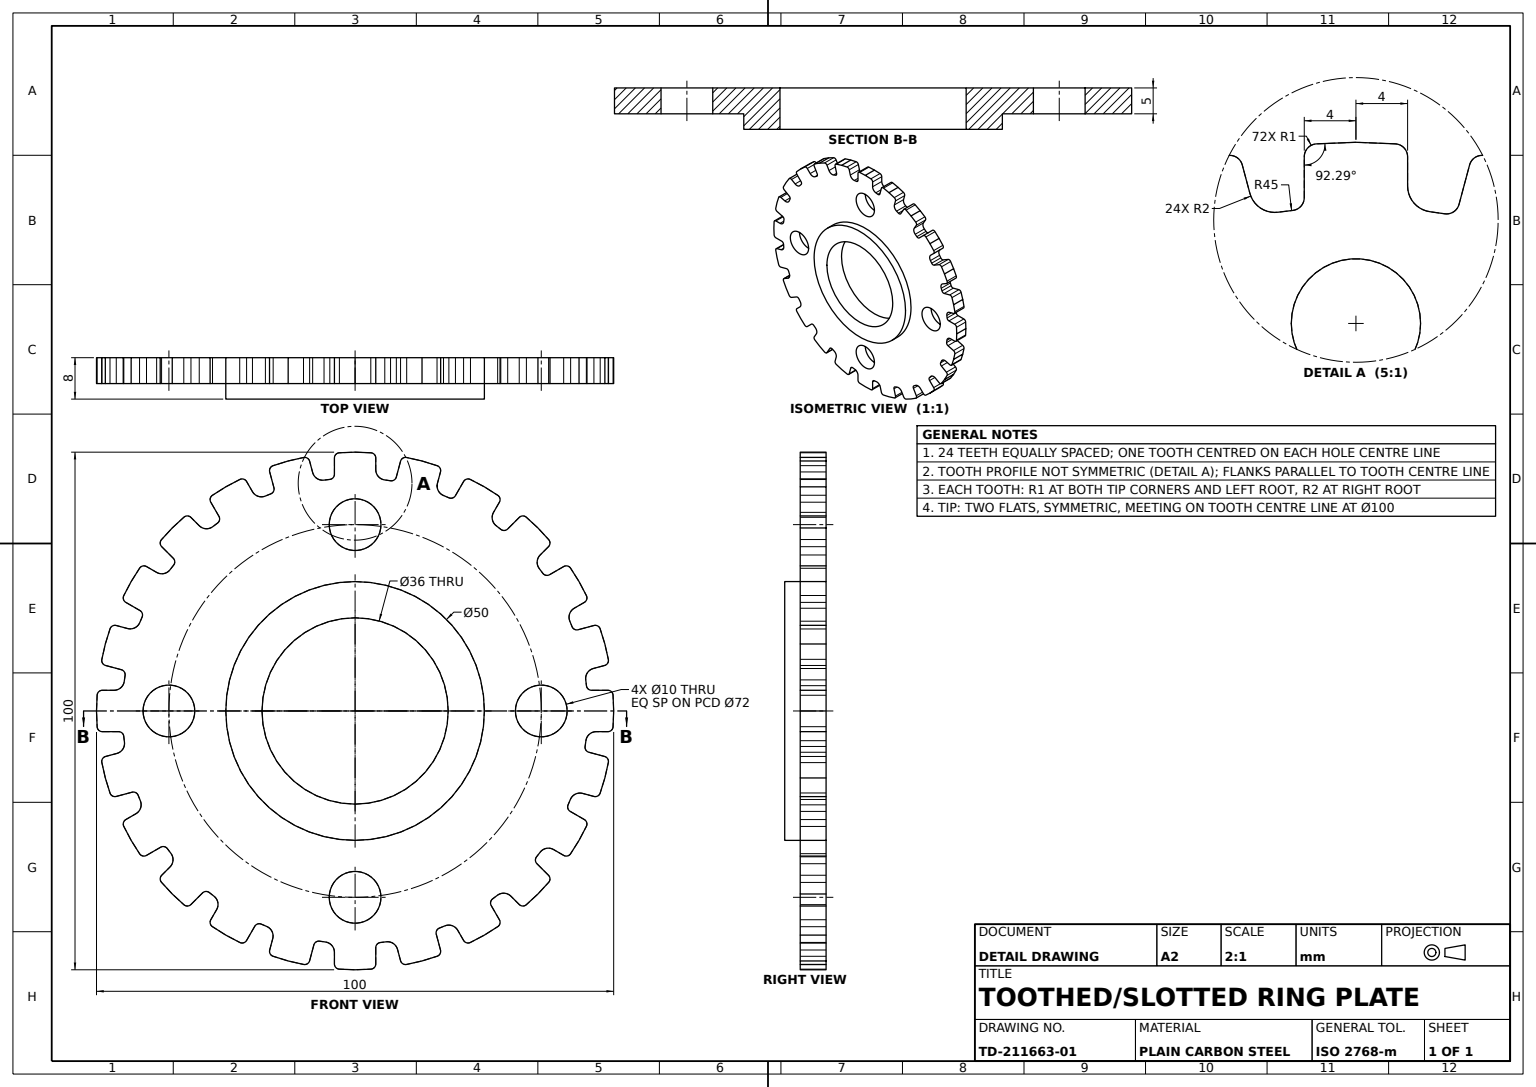
from build123d import *

# Parameters (mm, degrees)
TOOTHED_FLANGE_PLATE_24T_DEPTH     = 5
HUB_RING_SKETCH_R                  = 25
HUB_RING_SKETCH_R_2                = 18
HUB_RING_50_DEPTH                  = 3
CENTRE_BORE_SKETCH_R               = 18
CENTRE_BORE_DEPTH                  = 71.887234394
BOLT_HOLE_SKETCH_R                 = 5
BOLT_HOLE_10_DEPTH                 = 71.887234394
BOLT_HOLE_AND_HUB_PATTERN_4X_COUNT = 4


with BuildPart() as part:
    # Toothed Plate Profile Sketch → Toothed Flange Plate 24T (new body)
    with BuildSketch(Plane.XY):
        with BuildLine():
            Line((0, 50), (-3.036798719, 49.878430757))
            ThreePointArc((-3.036798719, 49.878430757), (-3.717908974, 49.5720514), (-3.996798719, 48.879231077))
            Line((-3.996798719, 48.879231077), (-3.996798719, 45.727803387))
            ThreePointArc((-3.996798719, 45.727803387), (-4.252276705, 45.060205476), (-4.88817266, 44.733720704))
            ThreePointArc((-4.88817266, 44.733720704), (-5.447357554, 44.669075384), (-6.00569006, 44.597440363))
            ThreePointArc((-6.00569006, 44.597440363), (-7.38128815, 44.91496722), (-8.204461271, 46.061910733))
            Line((-8.204461271, 46.061910733), (-8.790264808, 48.248159295))
            ThreePointArc((-8.790264808, 48.248159295), (-9.238966709, 48.84519036), (-9.976165508, 48.964845787))
            Line((-9.976165508, 48.964845787), (-12.940952255, 48.296291314))
            Line((-12.940952255, 48.296291314), (-15.842810132, 47.392883098))
            ThreePointArc((-15.842810132, 47.392883098), (-16.421415305, 46.920659059), (-16.511487018, 46.179264039))
            Line((-16.511487018, 46.179264039), (-15.695837512, 43.135218643))
            ThreePointArc((-15.695837512, 43.135218643), (-15.769823243, 42.424246011), (-16.299551092, 41.944303954))
            ThreePointArc((-16.299551092, 41.944303954), (-16.822950783, 41.737133669), (-17.343718063, 41.523432466))
            ThreePointArc((-17.343718063, 41.523432466), (-18.754625782, 41.474108874), (-19.846600784, 42.368918353))
            Line((-19.846600784, 42.368918353), (-20.978286314, 44.32905519))
            ThreePointArc((-20.978286314, 44.32905519), (-21.56622208, 44.789610317), (-22.309270542, 44.714387496))
            Line((-22.309270542, 44.714387496), (-25, 43.301270189))
            Line((-25, 43.301270189), (-27.569160215, 41.677588777))
            ThreePointArc((-27.569160215, 41.677588777), (-28.005829321, 41.071701343), (-27.900944763, 40.332256471))
            Line((-27.900944763, 40.332256471), (-26.325230918, 37.603040033))
            ThreePointArc((-26.325230918, 37.603040033), (-26.212682388, 36.897144289), (-26.600142054, 36.296452206))
            ThreePointArc((-26.600142054, 36.296452206), (-27.052087718, 35.960875269), (-27.499800341, 35.619671268))
            ThreePointArc((-27.499800341, 35.619671268), (-28.849866661, 35.206858548), (-30.136227252, 35.788554206))
            Line((-30.136227252, 35.788554206), (-31.736672277, 37.388999231))
            ThreePointArc((-31.736672277, 37.388999231), (-32.423775055, 37.68169235), (-33.122035656, 37.41671759))
            Line((-33.122035656, 37.41671759), (-35.355339059, 35.355339059))
            Line((-35.355339059, 35.355339059), (-37.41671759, 33.122035656))
            ThreePointArc((-37.41671759, 33.122035656), (-37.68169235, 32.423775055), (-37.388999231, 31.736672277))
            Line((-37.388999231, 31.736672277), (-35.160603341, 29.508276386))
            ThreePointArc((-35.160603341, 29.508276386), (-34.869190547, 28.85556316), (-35.087977293, 28.175057222))
            ThreePointArc((-35.087977293, 28.175057222), (-35.43766958, 27.733942647), (-35.781816671, 27.288488337))
            ThreePointArc((-35.781816671, 27.288488337), (-36.979036803, 26.540318993), (-38.372119634, 26.769259233))
            Line((-38.372119634, 26.769259233), (-40.332256471, 27.900944763))
            ThreePointArc((-40.332256471, 27.900944763), (-41.071701343, 28.005829321), (-41.677588777, 27.569160215))
            Line((-41.677588777, 27.569160215), (-43.301270189, 25))
            Line((-43.301270189, 25), (-44.714387496, 22.309270542))
            ThreePointArc((-44.714387496, 22.309270542), (-44.789610317, 21.56622208), (-44.32905519, 20.978286314))
            Line((-44.32905519, 20.978286314), (-41.599838752, 19.402572469))
            ThreePointArc((-41.599838752, 19.402572469), (-41.149420994, 18.847523088), (-41.184624866, 18.133578651))
            ThreePointArc((-41.184624866, 18.133578651), (-41.408232823, 17.616987667), (-41.625361328, 17.097640022))
            ThreePointArc((-41.625361328, 17.097640022), (-42.588146698, 16.065100559), (-43.993015477, 15.925683481))
            Line((-43.993015477, 15.925683481), (-46.179264039, 16.511487018))
            ThreePointArc((-46.179264039, 16.511487018), (-46.920659059, 16.421415305), (-47.392883098, 15.842810132))
            Line((-47.392883098, 15.842810132), (-48.296291314, 12.940952255))
            Line((-48.296291314, 12.940952255), (-48.964845787, 9.976165508))
            ThreePointArc((-48.964845787, 9.976165508), (-48.84519036, 9.238966709), (-48.248159295, 8.790264808))
            Line((-48.248159295, 8.790264808), (-45.204113898, 7.974615302))
            ThreePointArc((-45.204113898, 7.974615302), (-44.625386403, 7.555055464), (-44.474608314, 6.856326661))
            ThreePointArc((-44.474608314, 6.856326661), (-44.556893431, 6.29946409), (-44.632206399, 5.741615795))
            ThreePointArc((-44.632206399, 5.741615795), (-45.294944775, 4.495072071), (-46.615860017, 3.996798719))
            Line((-46.615860017, 3.996798719), (-48.879231077, 3.996798719))
            ThreePointArc((-48.879231077, 3.996798719), (-49.5720514, 3.717908974), (-49.878430757, 3.036798719))
            Line((-49.878430757, 3.036798719), (-50, 0))
            Line((-50, 0), (-49.878430757, -3.036798719))
            ThreePointArc((-49.878430757, -3.036798719), (-49.5720514, -3.717908974), (-48.879231077, -3.996798719))
            Line((-48.879231077, -3.996798719), (-45.727803387, -3.996798719))
            ThreePointArc((-45.727803387, -3.996798719), (-45.060205476, -4.252276705), (-44.733720704, -4.88817266))
            ThreePointArc((-44.733720704, -4.88817266), (-44.669075384, -5.447357554), (-44.597440363, -6.00569006))
            ThreePointArc((-44.597440363, -6.00569006), (-44.91496722, -7.38128815), (-46.061910733, -8.204461271))
            Line((-46.061910733, -8.204461271), (-48.248159295, -8.790264808))
            ThreePointArc((-48.248159295, -8.790264808), (-48.84519036, -9.238966709), (-48.964845787, -9.976165508))
            Line((-48.964845787, -9.976165508), (-48.296291314, -12.940952255))
            Line((-48.296291314, -12.940952255), (-47.392883098, -15.842810132))
            ThreePointArc((-47.392883098, -15.842810132), (-46.920659059, -16.421415305), (-46.179264039, -16.511487018))
            Line((-46.179264039, -16.511487018), (-43.135218643, -15.695837512))
            ThreePointArc((-43.135218643, -15.695837512), (-42.424246011, -15.769823243), (-41.944303954, -16.299551092))
            ThreePointArc((-41.944303954, -16.299551092), (-41.737133669, -16.822950783), (-41.523432466, -17.343718063))
            ThreePointArc((-41.523432466, -17.343718063), (-41.474108874, -18.754625782), (-42.368918353, -19.846600784))
            Line((-42.368918353, -19.846600784), (-44.32905519, -20.978286314))
            ThreePointArc((-44.32905519, -20.978286314), (-44.789610317, -21.56622208), (-44.714387496, -22.309270542))
            Line((-44.714387496, -22.309270542), (-43.301270189, -25))
            Line((-43.301270189, -25), (-41.677588777, -27.569160215))
            ThreePointArc((-41.677588777, -27.569160215), (-41.071701343, -28.005829321), (-40.332256471, -27.900944763))
            Line((-40.332256471, -27.900944763), (-37.603040033, -26.325230918))
            ThreePointArc((-37.603040033, -26.325230918), (-36.897144289, -26.212682388), (-36.296452206, -26.600142054))
            ThreePointArc((-36.296452206, -26.600142054), (-35.960875269, -27.052087718), (-35.619671268, -27.499800341))
            ThreePointArc((-35.619671268, -27.499800341), (-35.206858548, -28.849866661), (-35.788554206, -30.136227252))
            Line((-35.788554206, -30.136227252), (-37.388999231, -31.736672277))
            ThreePointArc((-37.388999231, -31.736672277), (-37.68169235, -32.423775055), (-37.41671759, -33.122035656))
            Line((-37.41671759, -33.122035656), (-35.355339059, -35.355339059))
            Line((-35.355339059, -35.355339059), (-33.122035656, -37.41671759))
            ThreePointArc((-33.122035656, -37.41671759), (-32.423775055, -37.68169235), (-31.736672277, -37.388999231))
            Line((-31.736672277, -37.388999231), (-29.508276386, -35.160603341))
            ThreePointArc((-29.508276386, -35.160603341), (-28.85556316, -34.869190547), (-28.175057222, -35.087977293))
            ThreePointArc((-28.175057222, -35.087977293), (-27.733942647, -35.43766958), (-27.288488337, -35.781816671))
            ThreePointArc((-27.288488337, -35.781816671), (-26.540318993, -36.979036803), (-26.769259233, -38.372119634))
            Line((-26.769259233, -38.372119634), (-27.900944763, -40.332256471))
            ThreePointArc((-27.900944763, -40.332256471), (-28.005829321, -41.071701343), (-27.569160215, -41.677588777))
            Line((-27.569160215, -41.677588777), (-25, -43.301270189))
            Line((-25, -43.301270189), (-22.309270542, -44.714387496))
            ThreePointArc((-22.309270542, -44.714387496), (-21.56622208, -44.789610317), (-20.978286314, -44.32905519))
            Line((-20.978286314, -44.32905519), (-19.402572469, -41.599838752))
            ThreePointArc((-19.402572469, -41.599838752), (-18.847523088, -41.149420994), (-18.133578651, -41.184624866))
            ThreePointArc((-18.133578651, -41.184624866), (-17.616987667, -41.408232823), (-17.097640022, -41.625361328))
            ThreePointArc((-17.097640022, -41.625361328), (-16.065100559, -42.588146698), (-15.925683481, -43.993015477))
            Line((-15.925683481, -43.993015477), (-16.511487018, -46.179264039))
            ThreePointArc((-16.511487018, -46.179264039), (-16.421415305, -46.920659059), (-15.842810132, -47.392883098))
            Line((-15.842810132, -47.392883098), (-12.940952255, -48.296291314))
            Line((-12.940952255, -48.296291314), (-9.976165508, -48.964845787))
            ThreePointArc((-9.976165508, -48.964845787), (-9.238966709, -48.84519036), (-8.790264808, -48.248159295))
            Line((-8.790264808, -48.248159295), (-7.974615302, -45.204113898))
            ThreePointArc((-7.974615302, -45.204113898), (-7.555055464, -44.625386403), (-6.856326661, -44.474608314))
            ThreePointArc((-6.856326661, -44.474608314), (-6.29946409, -44.556893431), (-5.741615795, -44.632206399))
            ThreePointArc((-5.741615795, -44.632206399), (-4.495072071, -45.294944775), (-3.996798719, -46.615860017))
            Line((-3.996798719, -46.615860017), (-3.996798719, -48.879231077))
            ThreePointArc((-3.996798719, -48.879231077), (-3.717908974, -49.5720514), (-3.036798719, -49.878430757))
            Line((-3.036798719, -49.878430757), (0, -50))
            Line((0, -50), (3.036798719, -49.878430757))
            ThreePointArc((3.036798719, -49.878430757), (3.717908974, -49.5720514), (3.996798719, -48.879231077))
            Line((3.996798719, -48.879231077), (3.996798719, -45.727803387))
            ThreePointArc((3.996798719, -45.727803387), (4.252276705, -45.060205476), (4.88817266, -44.733720704))
            ThreePointArc((4.88817266, -44.733720704), (5.447357554, -44.669075384), (6.00569006, -44.597440363))
            ThreePointArc((6.00569006, -44.597440363), (7.38128815, -44.91496722), (8.204461271, -46.061910733))
            Line((8.204461271, -46.061910733), (8.790264808, -48.248159295))
            ThreePointArc((8.790264808, -48.248159295), (9.238966709, -48.84519036), (9.976165508, -48.964845787))
            Line((9.976165508, -48.964845787), (12.940952255, -48.296291314))
            Line((12.940952255, -48.296291314), (15.842810132, -47.392883098))
            ThreePointArc((15.842810132, -47.392883098), (16.421415305, -46.920659059), (16.511487018, -46.179264039))
            Line((16.511487018, -46.179264039), (15.695837512, -43.135218643))
            ThreePointArc((15.695837512, -43.135218643), (15.769823243, -42.424246011), (16.299551092, -41.944303954))
            ThreePointArc((16.299551092, -41.944303954), (16.822950783, -41.737133669), (17.343718063, -41.523432466))
            ThreePointArc((17.343718063, -41.523432466), (18.754625782, -41.474108874), (19.846600784, -42.368918353))
            Line((19.846600784, -42.368918353), (20.978286314, -44.32905519))
            ThreePointArc((20.978286314, -44.32905519), (21.56622208, -44.789610317), (22.309270542, -44.714387496))
            Line((22.309270542, -44.714387496), (25, -43.301270189))
            Line((25, -43.301270189), (27.569160215, -41.677588777))
            ThreePointArc((27.569160215, -41.677588777), (28.005829321, -41.071701343), (27.900944763, -40.332256471))
            Line((27.900944763, -40.332256471), (26.325230918, -37.603040033))
            ThreePointArc((26.325230918, -37.603040033), (26.212682388, -36.897144289), (26.600142054, -36.296452206))
            ThreePointArc((26.600142054, -36.296452206), (27.052087718, -35.960875269), (27.499800341, -35.619671268))
            ThreePointArc((27.499800341, -35.619671268), (28.849866661, -35.206858548), (30.136227252, -35.788554206))
            Line((30.136227252, -35.788554206), (31.736672277, -37.388999231))
            ThreePointArc((31.736672277, -37.388999231), (32.423775055, -37.68169235), (33.122035656, -37.41671759))
            Line((33.122035656, -37.41671759), (35.355339059, -35.355339059))
            Line((35.355339059, -35.355339059), (37.41671759, -33.122035656))
            ThreePointArc((37.41671759, -33.122035656), (37.68169235, -32.423775055), (37.388999231, -31.736672277))
            Line((37.388999231, -31.736672277), (35.160603341, -29.508276386))
            ThreePointArc((35.160603341, -29.508276386), (34.869190547, -28.85556316), (35.087977293, -28.175057222))
            ThreePointArc((35.087977293, -28.175057222), (35.43766958, -27.733942647), (35.781816671, -27.288488337))
            ThreePointArc((35.781816671, -27.288488337), (36.979036803, -26.540318993), (38.372119634, -26.769259233))
            Line((38.372119634, -26.769259233), (40.332256471, -27.900944763))
            ThreePointArc((40.332256471, -27.900944763), (41.071701343, -28.005829321), (41.677588777, -27.569160215))
            Line((41.677588777, -27.569160215), (43.301270189, -25))
            Line((43.301270189, -25), (44.714387496, -22.309270542))
            ThreePointArc((44.714387496, -22.309270542), (44.789610317, -21.56622208), (44.32905519, -20.978286314))
            Line((44.32905519, -20.978286314), (41.599838752, -19.402572469))
            ThreePointArc((41.599838752, -19.402572469), (41.149420994, -18.847523088), (41.184624866, -18.133578651))
            ThreePointArc((41.184624866, -18.133578651), (41.408232823, -17.616987667), (41.625361328, -17.097640022))
            ThreePointArc((41.625361328, -17.097640022), (42.588146698, -16.065100559), (43.993015477, -15.925683481))
            Line((43.993015477, -15.925683481), (46.179264039, -16.511487018))
            ThreePointArc((46.179264039, -16.511487018), (46.920659059, -16.421415305), (47.392883098, -15.842810132))
            Line((47.392883098, -15.842810132), (48.296291314, -12.940952255))
            Line((48.296291314, -12.940952255), (48.964845787, -9.976165508))
            ThreePointArc((48.964845787, -9.976165508), (48.84519036, -9.238966709), (48.248159295, -8.790264808))
            Line((48.248159295, -8.790264808), (45.204113898, -7.974615302))
            ThreePointArc((45.204113898, -7.974615302), (44.625386403, -7.555055464), (44.474608314, -6.856326661))
            ThreePointArc((44.474608314, -6.856326661), (44.556893431, -6.29946409), (44.632206399, -5.741615795))
            ThreePointArc((44.632206399, -5.741615795), (45.294944775, -4.495072071), (46.615860017, -3.996798719))
            Line((46.615860017, -3.996798719), (48.879231077, -3.996798719))
            ThreePointArc((48.879231077, -3.996798719), (49.5720514, -3.717908974), (49.878430757, -3.036798719))
            Line((49.878430757, -3.036798719), (50, 0))
            Line((50, 0), (49.878430757, 3.036798719))
            ThreePointArc((49.878430757, 3.036798719), (49.5720514, 3.717908974), (48.879231077, 3.996798719))
            Line((48.879231077, 3.996798719), (45.727803387, 3.996798719))
            ThreePointArc((45.727803387, 3.996798719), (45.060205476, 4.252276705), (44.733720704, 4.88817266))
            ThreePointArc((44.733720704, 4.88817266), (44.669075384, 5.447357554), (44.597440363, 6.00569006))
            ThreePointArc((44.597440363, 6.00569006), (44.91496722, 7.38128815), (46.061910733, 8.204461271))
            Line((46.061910733, 8.204461271), (48.248159295, 8.790264808))
            ThreePointArc((48.248159295, 8.790264808), (48.84519036, 9.238966709), (48.964845787, 9.976165508))
            Line((48.964845787, 9.976165508), (48.296291314, 12.940952255))
            Line((48.296291314, 12.940952255), (47.392883098, 15.842810132))
            ThreePointArc((47.392883098, 15.842810132), (46.920659059, 16.421415305), (46.179264039, 16.511487018))
            Line((46.179264039, 16.511487018), (43.135218643, 15.695837512))
            ThreePointArc((43.135218643, 15.695837512), (42.424246011, 15.769823243), (41.944303954, 16.299551092))
            ThreePointArc((41.944303954, 16.299551092), (41.737133669, 16.822950783), (41.523432466, 17.343718063))
            ThreePointArc((41.523432466, 17.343718063), (41.474108874, 18.754625782), (42.368918353, 19.846600784))
            Line((42.368918353, 19.846600784), (44.32905519, 20.978286314))
            ThreePointArc((44.32905519, 20.978286314), (44.789610317, 21.56622208), (44.714387496, 22.309270542))
            Line((44.714387496, 22.309270542), (43.301270189, 25))
            Line((43.301270189, 25), (41.677588777, 27.569160215))
            ThreePointArc((41.677588777, 27.569160215), (41.071701343, 28.005829321), (40.332256471, 27.900944763))
            Line((40.332256471, 27.900944763), (37.603040033, 26.325230918))
            ThreePointArc((37.603040033, 26.325230918), (36.897144289, 26.212682388), (36.296452206, 26.600142054))
            ThreePointArc((36.296452206, 26.600142054), (35.960875269, 27.052087718), (35.619671268, 27.499800341))
            ThreePointArc((35.619671268, 27.499800341), (35.206858548, 28.849866661), (35.788554206, 30.136227252))
            Line((35.788554206, 30.136227252), (37.388999231, 31.736672277))
            ThreePointArc((37.388999231, 31.736672277), (37.68169235, 32.423775055), (37.41671759, 33.122035656))
            Line((37.41671759, 33.122035656), (35.355339059, 35.355339059))
            Line((35.355339059, 35.355339059), (33.122035656, 37.41671759))
            ThreePointArc((33.122035656, 37.41671759), (32.423775055, 37.68169235), (31.736672277, 37.388999231))
            Line((31.736672277, 37.388999231), (29.508276386, 35.160603341))
            ThreePointArc((29.508276386, 35.160603341), (28.85556316, 34.869190547), (28.175057222, 35.087977293))
            ThreePointArc((28.175057222, 35.087977293), (27.733942647, 35.43766958), (27.288488337, 35.781816671))
            ThreePointArc((27.288488337, 35.781816671), (26.540318993, 36.979036803), (26.769259233, 38.372119634))
            Line((26.769259233, 38.372119634), (27.900944763, 40.332256471))
            ThreePointArc((27.900944763, 40.332256471), (28.005829321, 41.071701343), (27.569160215, 41.677588777))
            Line((27.569160215, 41.677588777), (25, 43.301270189))
            Line((25, 43.301270189), (22.309270542, 44.714387496))
            ThreePointArc((22.309270542, 44.714387496), (21.56622208, 44.789610317), (20.978286314, 44.32905519))
            Line((20.978286314, 44.32905519), (19.402572469, 41.599838752))
            ThreePointArc((19.402572469, 41.599838752), (18.847523088, 41.149420994), (18.133578651, 41.184624866))
            ThreePointArc((18.133578651, 41.184624866), (17.616987667, 41.408232823), (17.097640022, 41.625361328))
            ThreePointArc((17.097640022, 41.625361328), (16.065100559, 42.588146698), (15.925683481, 43.993015477))
            Line((15.925683481, 43.993015477), (16.511487018, 46.179264039))
            ThreePointArc((16.511487018, 46.179264039), (16.421415305, 46.920659059), (15.842810132, 47.392883098))
            Line((15.842810132, 47.392883098), (12.940952255, 48.296291314))
            Line((12.940952255, 48.296291314), (9.976165508, 48.964845787))
            ThreePointArc((9.976165508, 48.964845787), (9.238966709, 48.84519036), (8.790264808, 48.248159295))
            Line((8.790264808, 48.248159295), (7.974615302, 45.204113898))
            ThreePointArc((7.974615302, 45.204113898), (7.555055464, 44.625386403), (6.856326661, 44.474608314))
            ThreePointArc((6.856326661, 44.474608314), (6.29946409, 44.556893431), (5.741615795, 44.632206399))
            ThreePointArc((5.741615795, 44.632206399), (4.495072071, 45.294944775), (3.996798719, 46.615860017))
            Line((3.996798719, 46.615860017), (3.996798719, 48.879231077))
            ThreePointArc((3.996798719, 48.879231077), (3.717908974, 49.5720514), (3.036798719, 49.878430757))
            Line((3.036798719, 49.878430757), (0, 50))
        make_face()
    extrude(amount=TOOTHED_FLANGE_PLATE_24T_DEPTH)

    # Hub Ring Sketch → Hub Ring Ø50 (add)
    with BuildSketch(Plane.XY.offset(5)):
        Circle(HUB_RING_SKETCH_R)
        Circle(HUB_RING_SKETCH_R_2, mode=Mode.SUBTRACT)
    extrude(amount=HUB_RING_50_DEPTH)

    # Centre Bore Sketch → Centre Bore (cut, through all)
    with BuildSketch(Plane.XY.offset(5)):
        Circle(CENTRE_BORE_SKETCH_R)
    extrude(amount=-CENTRE_BORE_DEPTH, mode=Mode.SUBTRACT)

    # Bolt Hole Sketch → Bolt Hole Ø10 (cut, through all)
    with BuildSketch(Plane.XY.offset(5)):
        with Locations((0, 36)):
            Circle(BOLT_HOLE_SKETCH_R)
    bolt_hole_10 = extrude(amount=-BOLT_HOLE_10_DEPTH, mode=Mode.SUBTRACT)

    # Bolt Hole and Hub Pattern 4x: Bolt Hole Ø10 ×4 about axis
    bolt_hole_and_hub_pattern_4x_axis = Axis((0, 0, 0), (0, 0, 1))
    for i in range(1, BOLT_HOLE_AND_HUB_PATTERN_4X_COUNT):
        add(bolt_hole_10.rotate(bolt_hole_and_hub_pattern_4x_axis, i * 360 / BOLT_HOLE_AND_HUB_PATTERN_4X_COUNT), mode=Mode.SUBTRACT)


solid = part.part
